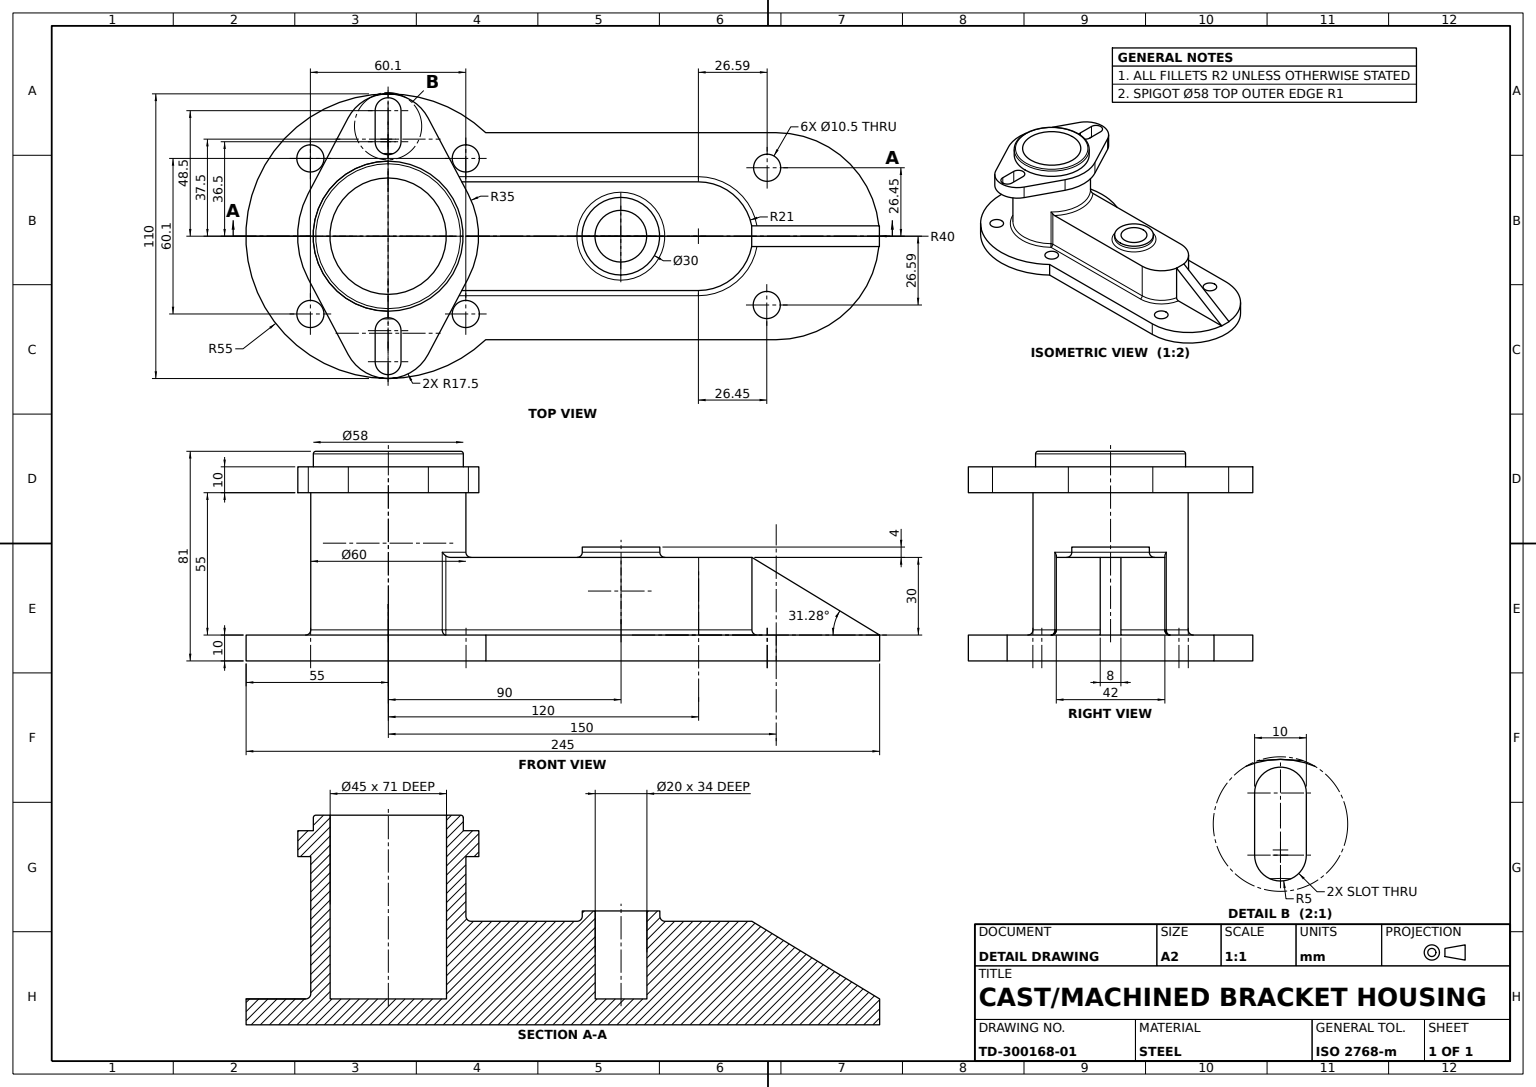
SolidWorks part; units mm, degrees
material "Plain Carbon Steel"
ref_plane "Front Plane" through (0, 0, 0) normal (0, 0, 1) x (1, 0, 0)
ref_plane "Top Plane" through (0, 0, 0) normal (0, 1, 0) x (1, 0, 0)
ref_plane "Right Plane" through (0, 0, 0) normal (1, 0, 0) x (0, 0, -1)
sketch "Base Plate Sketch" plane through (0, 0, 0) normal (0, 1, 0) x (1, 0, 0)
  line L2 (37.7492, 40) -> (150, 40)
  line L3 (37.7492, -40) -> (150, -40)
  arc A0 (37.7492, 40) -> (37.7492, -40) centre (0, 0) ccw
  arc A1 (150, -40) -> (150, 40) centre (150, 0) ccw
  dimension "D1" = 110
  dimension "D2" = 80
  dimension "D3" = 150
extrude "Base Plate" add sketch "Base Plate Sketch" along normal blind 10
sketch "Bearing Column Sketch" plane through (0, 10, 0) normal (0, 1, 0) x (1, 0, 0)
  circle A0 centre (0, 0) radius 30
  dimension "D1" = 60
extrude "Bearing Column Ø60" add sketch "Bearing Column Sketch" along normal blind 55
sketch "Top Flange Sketch" plane through (0, 65, 0) normal (0, 1, 0) x (1, 0, 0)
  line L0 (-15.4776, 45.6667) -> (-30.9552, 16.3333)
  line L1 (15.4776, 45.6667) -> (30.9552, 16.3333)
  line L2 (-30.9552, -16.3333) -> (-15.4776, -45.6667)
  line L3 (15.4776, -45.6667) -> (30.9552, -16.3333)
  arc A0 (-30.9552, 16.3333) -> (-30.9552, -16.3333) centre (0, 0) ccw
  arc A2 (15.4776, 45.6667) -> (-15.4776, 45.6667) centre (0, 37.5) ccw
  arc A3 (-15.4776, -45.6667) -> (15.4776, -45.6667) centre (0, -37.5) ccw
  arc A4 (30.9552, -16.3333) -> (30.9552, 16.3333) centre (0, 0) ccw
  dimension "D1" = 70
  dimension "D2" = 35
  dimension "D3" = 35
  dimension "D4" = 37.5
  dimension "D5" = 37.5
extrude "Top Flange" add sketch "Top Flange Sketch" along normal blind 10
sketch "Bearing Spigot Sketch" plane through (0, 75, 0) normal (0, 1, 0) x (1, 0, 0)
  circle A0 centre (0, 0) radius 29
  dimension "D1" = 58
extrude "Bearing Spigot Ø58" add sketch "Bearing Spigot Sketch" along normal blind 6
sketch "Bearing Bore Sketch" plane through (0, 81, 0) normal (0, 1, 0) x (1, 0, 0)
  circle A0 centre (0, 0) radius 22.5
  dimension "D1" = 45
extrude "Bearing Bore Ø45" cut sketch "Bearing Bore Sketch" against normal blind 61
sketch "Flange Slots Sketch" plane through (0, 75, 0) normal (0, 1, 0) x (1, 0, 0)
  line L0 (0, 36.5) -> (0, 48.5) construction
  line L1 (-5, 36.5) -> (-5, 48.5)
  line L2 (5, 36.5) -> (5, 48.5)
  line L3 (0, -36.5) -> (0, -48.5) construction
  line L4 (5, -36.5) -> (5, -48.5)
  line L5 (-5, -36.5) -> (-5, -48.5)
  arc A1 (-5, 36.5) -> (5, 36.5) centre (0, 36.5) ccw
  arc A2 (5, 48.5) -> (-5, 48.5) centre (0, 48.5) ccw
  arc A3 (5, -36.5) -> (-5, -36.5) centre (0, -36.5) ccw
  arc A4 (-5, -48.5) -> (5, -48.5) centre (0, -48.5) ccw
  point P5 (0, 42.5)
  point P12 (0, -42.5)
  dimension "D1" = 48.5
  dimension "D2" = 5
  dimension "D4" = 5
  dimension "D3" = 12
  dimension "D5" = 12
  dimension "D6" = 48.5
extrude "Flange Slots 2x" cut sketch "Flange Slots Sketch" against normal blind 10
sketch "Arm Block Sketch" plane through (0, 10, 0) normal (0, 1, 0) x (1, 0, 0)
  line L1 (120, 21) -> (20, 21)
  line L3 (120, -21) -> (20, -21)
  line L4 (20, 21) -> (20, -21)
  arc A0 (120, -21) -> (120, 21) centre (120, 0) ccw
  dimension "D1" = 42
  dimension "D2" = 120
  dimension "D3" = 42
  dimension "D4" = 20
  dimension "95" = 100
extrude "Arm Block" add sketch "Arm Block Sketch" along normal blind 30
sketch "Column Clearance Sketch" plane through (0, 40, 0) normal (0, 1, 0) x (1, 0, 0)
  circle A0 centre (0, 0) radius 22.5
  dimension "D1" = 45
extrude "Column Clearance Cut Ø45" cut sketch "Column Clearance Sketch" against normal blind 30
sketch "Arm Boss Sketch" plane through (0, 40, 0) normal (0, 1, 0) x (1, 0, 0)
  circle A0 centre (90, 0) radius 15
  dimension "D1" = 30
  dimension "D2" = 90
  dimension "D3" = 68.5757
extrude "Arm Boss Ø30" add sketch "Arm Boss Sketch" along normal blind 4
sketch "Arm Boss Bore Sketch" plane through (0, 44, 0) normal (0, 1, 0) x (1, 0, 0)
  circle A0 centre (90, 0) radius 10
  dimension "D1" = 20
extrude "Arm Boss Bore Ø20" cut sketch "Arm Boss Bore Sketch" against normal blind 34
sketch "Base Mounting Holes Sketch" plane through (0, 10, 0) normal (0, 1, 0) x (1, 0, 0)
  circle A1 centre (-30.052, 30.052) radius 5.25
  circle A2 centre (30.052, 30.052) radius 5.25
  circle A3 centre (30.052, -30.052) radius 5.25
  circle A4 centre (-30.052, -30.052) radius 5.25
  dimension "D1" = 30.052
  dimension "D3" = 10.5
  dimension "D2" = 4
  dimension "D4" = 60.1041
  dimension "D5" = 30.052
  dimension "D6" = 30.052
extrude "Base Mounting Holes 4xØ10.5" cut sketch "Base Mounting Holes Sketch" against normal blind 34
sketch "Base Diagonal Holes Sketch" plane through (0, 10, 0) normal (0, 1, 0) x (1, 0, 0)
  line L0 (120, 0) -> (120, 82.0498) construction
  line L1 (120, 0) -> (184.7718, 64.7718) construction
  circle A1 centre (146.5868, 26.446) radius 5.25
  circle A2 centre (146.446, -26.5868) radius 5.25
  dimension "D1" = 26.5868
  dimension "D3" = 10.5
  dimension "D2" = 45
  dimension "D5" = 26.5868
  dimension "D6" = 26.446
  dimension "D7" = 26.446
  dimension "D4" = 2
extrude "Base Diagonal Holes 2xØ10.5" cut sketch "Base Diagonal Holes Sketch" against normal blind 34
ref_plane "Rib Plane" through (140, 0, 0) normal (1, 0, 0) x (0, 0, -1)
sketch "Gusset Rib Sketch" plane through (140, 0, 0) normal (1, 0, 0) x (0, 0, -1)
  line L0 (21, 40) -> (-21, 40) construction
  line L1 (-4, 40) -> (4, 40)
  line L2 (-4, 40) -> (-4, 10)
  line L3 (-4, 10) -> (4, 10)
  line L4 (4, 40) -> (4, 10)
  line L5 (40, 10) -> (-40, 10) construction
  dimension "D1" = 4
  dimension "D2" = 8
extrude "Gusset Rib" add sketch "Gusset Rib Sketch" along normal blind 50
sketch "Rib Trim Sketch" plane through (0, 0, 4) normal (0, 0, 1) x (1, 0, 0)
  line L0 (140.6155, 40) -> (190, 10)
extrude "Rib Trim Cut" cut sketch "Rib Trim Sketch" against normal blind 49.8 and the other way through all
fillet "Column-Arm Fillet R2" radius 2 3 edges at (21.4243, 25, 21) (21.4243, 25, -21) (30, 40, 0)
fillet "Column-Base Fillet R2" radius 2 7 edges at (133.3604, 10, -16.2019) (71.1243, 10, -21) (21.4986, 10, -21.146) (133.3604, 10, 16.2019) (71.1243, 10, 21) (21.4986, 10, 21.146) (-30, 10, 0)
fillet "Arm Boss Fillet R2" radius 2 1 edges at (90, 40, 15)
fillet "Spigot Fillet R1" radius 1 1 edges at (0, 81, 29)
